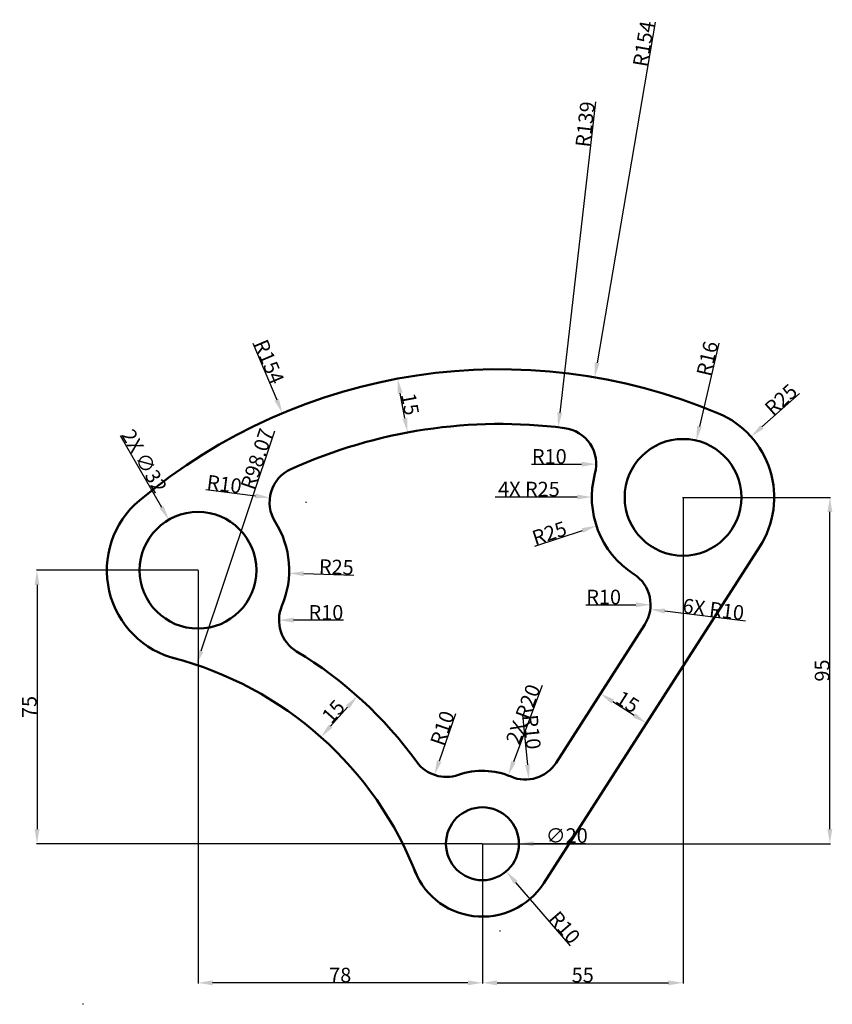
# Model space of a CAD drawing. Units: millimetres. Extents: x 51 to 274, y 49 to 320.
import ezdxf

# ---------------------------------------------------------------- set-up
doc = ezdxf.new("R2010")
doc.units = ezdxf.units.MM
doc.header["$MEASUREMENT"] = 0
doc.layers.add('M-DIMS', color=2, linetype='Continuous', lineweight=25)
doc.layers.add('M-OUTL', color=7, linetype='Continuous', lineweight=50)
doc.styles.get("Standard").update_dxf_attribs({"font": 'arial.ttf'})
doc.dimstyles.get("Standard").update_dxf_attribs({"dimtxt": 4, "dimasz": 4, "dimexe": 0.18, "dimexo": 0.0625, "dimgap": 0.09, "dimtad": 1, "dimdec": 0, "dimzin": 0, "dimdsep": 46, "dimtxsty": 'Standard', "dimcen": 0.09, "dimclre": 251, "dimadec": 0, "dimazin": 0, "dimtfac": 1, "dimtdec": 0, "dimtofl": 0, "dimtmove": 0, "dimatfit": 3, "dimfxl": 1, "dimtolj": 1, "dimtzin": 0, "dimarcsym": 0})

# ---------------------------------------------------------------- blocks, each defined once
blk = doc.blocks.new('*D1')
at = {"layer": 'Defpoints', "color": 0, "transparency": 16777216}
for p in [(233.24, 188.51), (178.24, 93.51), (233.24, 55.36)]:
    blk.add_point(p, dxfattribs=at)
at = {"layer": 'M-DIMS', "color": 0, "lineweight": -2, "transparency": 16777216}
for p, q in [((233.24, 188.45), (233.24, 55.18)), ((178.24, 93.45), (178.24, 55.18)), ((182.24, 55.36), (229.24, 55.36))]:
    blk.add_line(p, q, dxfattribs=at)
at = {"layer": 'M-DIMS', "color": 0, "transparency": 16777216}
for points in [[(182.24, 56.02), (182.24, 54.69), (178.24, 55.36)], [(229.24, 56.02), (229.24, 54.69), (233.24, 55.36)]]:
    blk.add_solid(points, dxfattribs=at)
at = {"layer": 'M-DIMS', "color": 0, "transparency": 16777216, "insert": (205.74, 57.48), "char_height": 4, "attachment_point": 5}
blk.add_mtext('\\A1;55', dxfattribs=at)
blk = doc.blocks.new('*D2')
at = {"layer": 'Defpoints', "color": 0, "transparency": 16777216}
for p in [(100.24, 168.51), (178.24, 93.51), (100.24, 55.36)]:
    blk.add_point(p, dxfattribs=at)
at = {"layer": 'M-DIMS', "color": 0, "lineweight": -2, "transparency": 16777216}
for p, q in [((100.24, 168.45), (100.24, 55.18)), ((178.24, 93.45), (178.24, 55.18)), ((174.24, 55.36), (104.24, 55.36))]:
    blk.add_line(p, q, dxfattribs=at)
at = {"layer": 'M-DIMS', "color": 0, "transparency": 16777216}
for points in [[(104.24, 56.02), (104.24, 54.69), (100.24, 55.36)], [(174.24, 56.02), (174.24, 54.69), (178.24, 55.36)]]:
    blk.add_solid(points, dxfattribs=at)
at = {"layer": 'M-DIMS', "color": 0, "transparency": 16777216, "insert": (139.24, 57.49), "char_height": 4, "attachment_point": 5}
blk.add_mtext('\\A1;78', dxfattribs=at)
blk = doc.blocks.new('*D3')
at = {"layer": 'Defpoints', "color": 0, "transparency": 16777216}
for p in [(233.24, 188.51), (273.51, 188.51), (178.24, 93.51)]:
    blk.add_point(p, dxfattribs=at)
at = {"layer": 'M-DIMS', "color": 0, "lineweight": -2, "transparency": 16777216}
for p, q in [((233.3, 188.51), (273.69, 188.51)), ((273.51, 97.51), (273.51, 184.51)), ((178.3, 93.51), (273.69, 93.51))]:
    blk.add_line(p, q, dxfattribs=at)
at = {"layer": 'M-DIMS', "color": 0, "transparency": 16777216}
for points in [[(272.84, 184.51), (274.18, 184.51), (273.51, 188.51)], [(272.84, 97.51), (274.18, 97.51), (273.51, 93.51)]]:
    blk.add_solid(points, dxfattribs=at)
at = {"layer": 'M-DIMS', "color": 0, "transparency": 16777216, "insert": (271.38, 141.01), "char_height": 4, "attachment_point": 5, "rotation": 90}
blk.add_mtext('\\A1;95', dxfattribs=at)
blk = doc.blocks.new('*D4')
at = {"layer": 'Defpoints', "color": 0, "transparency": 16777216}
for p in [(100.24, 168.51), (56.09, 93.51), (178.24, 93.51)]:
    blk.add_point(p, dxfattribs=at)
at = {"layer": 'M-DIMS', "color": 0, "lineweight": -2, "transparency": 16777216}
for p, q in [((100.18, 168.51), (55.91, 168.51)), ((56.09, 164.51), (56.09, 97.51)), ((178.18, 93.51), (55.91, 93.51))]:
    blk.add_line(p, q, dxfattribs=at)
at = {"layer": 'M-DIMS', "color": 0, "transparency": 16777216}
for points in [[(55.43, 164.51), (56.76, 164.51), (56.09, 168.51)], [(55.43, 97.51), (56.76, 97.51), (56.09, 93.51)]]:
    blk.add_solid(points, dxfattribs=at)
at = {"layer": 'M-DIMS', "color": 0, "transparency": 16777216, "insert": (53.97, 131.01), "char_height": 4, "attachment_point": 5, "rotation": 90}
blk.add_mtext('\\A1;75', dxfattribs=at)
blk = doc.blocks.new('*D5')
at = {"layer": 'Defpoints', "color": 0, "transparency": 16777216}
for p in [(143.92, 133.98), (143.92, 133.98), (133.95, 122.78)]:
    blk.add_point(p, dxfattribs=at)
at = {"layer": 'M-DIMS', "color": 0, "lineweight": -2, "transparency": 16777216}
for p, q in [((143.97, 133.94), (144.06, 133.86)), ((136.61, 125.77), (141.26, 130.99)), ((133.99, 122.74), (134.08, 122.66))]:
    blk.add_line(p, q, dxfattribs=at)
at = {"layer": 'M-DIMS', "color": 0, "transparency": 16777216}
for points in [[(140.77, 131.44), (141.76, 130.55), (143.92, 133.98)], [(136.11, 126.21), (137.11, 125.32), (133.95, 122.78)]]:
    blk.add_solid(points, dxfattribs=at)
at = {"layer": 'M-DIMS', "color": 0, "transparency": 16777216, "insert": (137.34, 129.8), "char_height": 4, "attachment_point": 5, "rotation": 48.3021}
blk.add_mtext('\\A1;15', dxfattribs=at)
blk = doc.blocks.new('*D6')
at = {"layer": 'Defpoints', "color": 0, "transparency": 16777216}
for p in [(154.95, 221.05), (154.95, 221.05), (157.7, 206.31)]:
    blk.add_point(p, dxfattribs=at)
at = {"layer": 'M-DIMS', "color": 0, "lineweight": -2, "transparency": 16777216}
for p, q in [((154.89, 221.04), (154.78, 221.02)), ((156.97, 210.24), (155.69, 217.12)), ((157.64, 206.29), (157.52, 206.27))]:
    blk.add_line(p, q, dxfattribs=at)
at = {"layer": 'M-DIMS', "color": 0, "transparency": 16777216}
for points in [[(156.34, 217.24), (155.03, 217), (154.95, 221.05)], [(157.62, 210.36), (156.31, 210.12), (157.7, 206.31)]]:
    blk.add_solid(points, dxfattribs=at)
at = {"layer": 'M-DIMS', "color": 0, "transparency": 16777216, "insert": (158.42, 214.07), "char_height": 4, "attachment_point": 5, "rotation": 280.5338}
blk.add_mtext('\\A1;15', dxfattribs=at)
blk = doc.blocks.new('*D7')
at = {"layer": 'Defpoints', "color": 0, "transparency": 16777216}
for p in [(210.59, 134.68), (223.21, 126.58), (223.21, 126.58)]:
    blk.add_point(p, dxfattribs=at)
at = {"layer": 'M-DIMS', "color": 0, "lineweight": -2, "transparency": 16777216}
for p, q in [((210.62, 134.73), (210.68, 134.83)), ((213.95, 132.52), (219.85, 128.74)), ((223.25, 126.63), (223.31, 126.73))]:
    blk.add_line(p, q, dxfattribs=at)
at = {"layer": 'M-DIMS', "color": 0, "transparency": 16777216}
for points in [[(214.31, 133.08), (213.59, 131.96), (210.59, 134.68)], [(220.21, 129.3), (219.49, 128.18), (223.21, 126.58)]]:
    blk.add_solid(points, dxfattribs=at)
at = {"layer": 'M-DIMS', "color": 0, "transparency": 16777216, "insert": (218.05, 132.42), "char_height": 4, "attachment_point": 5, "rotation": 327.3208}
blk.add_mtext('\\A1;15', dxfattribs=at)
blk = doc.blocks.new('*D8')
at = {"layer": 'Defpoints', "color": 0, "transparency": 16777216}
for p in [(251.89, 205.15), (233.24, 188.51)]:
    blk.add_point(p, dxfattribs=at)
at = {"layer": 'M-DIMS', "color": 0, "lineweight": -2, "transparency": 16777216}
for p, q in [((265.15, 216.98), (254.88, 207.82)), ((233.15, 188.51), (233.33, 188.51)), ((233.24, 188.42), (233.24, 188.6))]:
    blk.add_line(p, q, dxfattribs=at)
at = {"layer": 'M-DIMS', "color": 0, "transparency": 16777216}
blk.add_solid([(254.43, 208.31), (255.32, 207.32), (251.89, 205.15)], dxfattribs=at)
at = {"layer": 'M-DIMS', "color": 0, "transparency": 16777216, "insert": (260.09, 215.32), "char_height": 4, "attachment_point": 5, "rotation": 41.7376}
blk.add_mtext('\\A1;R25', dxfattribs=at)
blk = doc.blocks.new('*D9')
at = {"layer": 'Defpoints', "color": 0, "transparency": 16777216}
for p in [(236.86, 204.09), (233.24, 188.51)]:
    blk.add_point(p, dxfattribs=at)
at = {"layer": 'M-DIMS', "color": 0, "lineweight": -2, "transparency": 16777216}
for p, q in [((243.07, 230.83), (237.76, 207.99)), ((233.15, 188.51), (233.33, 188.51)), ((233.24, 188.42), (233.24, 188.6))]:
    blk.add_line(p, q, dxfattribs=at)
at = {"layer": 'M-DIMS', "color": 0, "transparency": 16777216}
blk.add_solid([(237.11, 208.14), (238.41, 207.84), (236.86, 204.09)], dxfattribs=at)
at = {"layer": 'M-DIMS', "color": 0, "transparency": 16777216, "insert": (239.89, 226.57), "char_height": 4, "attachment_point": 5, "rotation": 76.92}
blk.add_mtext('\\A1;R16', dxfattribs=at)
blk = doc.blocks.new('*D10')
at = {"layer": 'Defpoints', "color": 0, "transparency": 16777216}
for p in [(233.24, 188.51), (209.49, 180.71)]:
    blk.add_point(p, dxfattribs=at)
at = {"layer": 'M-DIMS', "color": 0, "lineweight": -2, "transparency": 16777216}
for p, q in [((233.15, 188.51), (233.33, 188.51)), ((233.24, 188.42), (233.24, 188.6)), ((192.61, 175.16), (205.69, 179.46))]:
    blk.add_line(p, q, dxfattribs=at)
at = {"layer": 'M-DIMS', "color": 0, "transparency": 16777216}
blk.add_solid([(205.48, 180.09), (205.89, 178.82), (209.49, 180.71)], dxfattribs=at)
at = {"layer": 'M-DIMS', "color": 0, "transparency": 16777216, "insert": (196.58, 178.71), "char_height": 4, "attachment_point": 5, "rotation": 18.1877}
blk.add_mtext('\\A1;R25', dxfattribs=at)
blk = doc.blocks.new('*D11')
at = {"layer": 'Defpoints', "color": 0, "transparency": 16777216}
for p in [(100.24, 168.51), (125.22, 167.7)]:
    blk.add_point(p, dxfattribs=at)
at = {"layer": 'M-DIMS', "color": 0, "lineweight": -2, "transparency": 16777216}
for p, q in [((100.15, 168.51), (100.33, 168.51)), ((100.24, 168.42), (100.24, 168.6)), ((142.98, 167.12), (129.22, 167.57))]:
    blk.add_line(p, q, dxfattribs=at)
at = {"layer": 'M-DIMS', "color": 0, "transparency": 16777216}
blk.add_solid([(129.24, 168.23), (129.2, 166.9), (125.22, 167.7)], dxfattribs=at)
at = {"layer": 'M-DIMS', "color": 0, "transparency": 16777216, "insert": (138.17, 169.41), "char_height": 4, "attachment_point": 5, "rotation": 358.1393}
blk.add_mtext('\\A1;R25', dxfattribs=at)
blk = doc.blocks.new('*D12')
at = {"layer": 'Defpoints', "color": 0, "transparency": 16777216}
for p in [(119.94, 188.41), (129.86, 187.15)]:
    blk.add_point(p, dxfattribs=at)
at = {"layer": 'M-DIMS', "color": 0, "lineweight": -2, "transparency": 16777216}
for p, q in [((102.36, 190.64), (115.97, 188.91)), ((129.77, 187.15), (129.95, 187.15)), ((129.86, 187.06), (129.86, 187.24))]:
    blk.add_line(p, q, dxfattribs=at)
at = {"layer": 'M-DIMS', "color": 0, "transparency": 16777216}
blk.add_solid([(116.06, 189.57), (115.89, 188.25), (119.94, 188.41)], dxfattribs=at)
at = {"layer": 'M-DIMS', "color": 0, "transparency": 16777216, "insert": (107.45, 192.14), "char_height": 4, "attachment_point": 5, "rotation": 352.7636}
blk.add_mtext('\\A1;R10', dxfattribs=at)
blk = doc.blocks.new('*D13')
at = {"layer": 'Defpoints', "color": 0, "transparency": 16777216}
for p in [(199.44, 197.61), (209.44, 197.61)]:
    blk.add_point(p, dxfattribs=at)
at = {"layer": 'M-DIMS', "color": 0, "lineweight": -2, "transparency": 16777216}
blk.add_line((191.72, 197.61), (205.44, 197.61), dxfattribs=at)
at = {"layer": 'M-DIMS', "color": 0, "transparency": 16777216}
blk.add_solid([(205.44, 198.28), (205.44, 196.94), (209.44, 197.61)], dxfattribs=at)
at = {"layer": 'M-DIMS', "color": 0, "transparency": 16777216, "insert": (196.58, 199.74), "char_height": 4, "attachment_point": 5}
blk.add_mtext('\\A1;R10', dxfattribs=at)
blk = doc.blocks.new('*D14')
at = {"layer": 'Defpoints', "color": 0, "transparency": 16777216}
for p in [(214.34, 159.05), (224.34, 159.05)]:
    blk.add_point(p, dxfattribs=at)
at = {"layer": 'M-DIMS', "color": 0, "lineweight": -2, "transparency": 16777216}
blk.add_line((206.62, 159.05), (220.34, 159.05), dxfattribs=at)
at = {"layer": 'M-DIMS', "color": 0, "transparency": 16777216}
blk.add_solid([(220.34, 159.72), (220.34, 158.38), (224.34, 159.05)], dxfattribs=at)
at = {"layer": 'M-DIMS', "color": 0, "transparency": 16777216, "insert": (211.48, 161.18), "char_height": 4, "attachment_point": 5}
blk.add_mtext('\\A1;R10', dxfattribs=at)
blk = doc.blocks.new('*D15')
at = {"layer": 'Defpoints', "color": 0, "transparency": 16777216}
for p in [(190, 121.11), (190.97, 111.15)]:
    blk.add_point(p, dxfattribs=at)
at = {"layer": 'M-DIMS', "color": 0, "lineweight": -2, "transparency": 16777216}
blk.add_line((189.25, 128.8), (190.58, 115.14), dxfattribs=at)
at = {"layer": 'M-DIMS', "color": 0, "transparency": 16777216}
blk.add_solid([(191.24, 115.2), (189.92, 115.07), (190.97, 111.15)], dxfattribs=at)
at = {"layer": 'M-DIMS', "color": 0, "transparency": 16777216, "insert": (191.85, 124.16), "char_height": 4, "attachment_point": 5, "rotation": 275.5492}
blk.add_mtext('\\A1;R10', dxfattribs=at)
blk = doc.blocks.new('*D16')
at = {"layer": 'Defpoints', "color": 0, "transparency": 16777216}
for p in [(168.33, 121.82), (165.08, 112.37)]:
    blk.add_point(p, dxfattribs=at)
at = {"layer": 'M-DIMS', "color": 0, "lineweight": -2, "transparency": 16777216}
blk.add_line((170.84, 129.13), (166.38, 116.15), dxfattribs=at)
at = {"layer": 'M-DIMS', "color": 0, "transparency": 16777216}
blk.add_solid([(165.75, 116.37), (167.01, 115.93), (165.08, 112.37)], dxfattribs=at)
at = {"layer": 'M-DIMS', "color": 0, "transparency": 16777216, "insert": (167.24, 125.22), "char_height": 4, "attachment_point": 5, "rotation": 71.0428}
blk.add_mtext('\\A1;R10', dxfattribs=at)
blk = doc.blocks.new('*D17')
at = {"layer": 'Defpoints', "color": 0, "transparency": 16777216}
for p in [(122.45, 154.83), (132.45, 154.83)]:
    blk.add_point(p, dxfattribs=at)
at = {"layer": 'M-DIMS', "color": 0, "lineweight": -2, "transparency": 16777216}
blk.add_line((140.18, 154.83), (126.45, 154.83), dxfattribs=at)
at = {"layer": 'M-DIMS', "color": 0, "transparency": 16777216}
blk.add_solid([(126.45, 155.5), (126.45, 154.16), (122.45, 154.83)], dxfattribs=at)
at = {"layer": 'M-DIMS', "color": 0, "transparency": 16777216, "insert": (135.32, 156.96), "char_height": 4, "attachment_point": 5}
blk.add_mtext('\\A1;R10', dxfattribs=at)
blk = doc.blocks.new('*D18')
at = {"layer": 'Defpoints', "color": 0, "transparency": 16777216}
for p in [(123.37, 211.59), (183.11, 69.65)]:
    blk.add_point(p, dxfattribs=at)
at = {"layer": 'M-DIMS', "color": 0, "lineweight": -2, "transparency": 16777216}
for p, q in [((115.29, 230.79), (121.82, 215.27)), ((183.02, 69.65), (183.2, 69.65)), ((183.11, 69.56), (183.11, 69.74))]:
    blk.add_line(p, q, dxfattribs=at)
at = {"layer": 'M-DIMS', "color": 0, "transparency": 16777216}
blk.add_solid([(122.43, 215.53), (121.2, 215.02), (123.37, 211.59)], dxfattribs=at)
at = {"layer": 'M-DIMS', "color": 0, "transparency": 16777216, "insert": (119.74, 225.7), "char_height": 4, "attachment_point": 5, "rotation": 292.8258}
blk.add_mtext('\\A1;R154', dxfattribs=at)
blk = doc.blocks.new('*D19')
at = {"layer": 'Defpoints', "color": 0, "transparency": 16777216}
for p in [(178.24, 93.51), (184.75, 85.92)]:
    blk.add_point(p, dxfattribs=at)
at = {"layer": 'M-DIMS', "color": 0, "lineweight": -2, "transparency": 16777216}
for p, q in [((178.15, 93.51), (178.33, 93.51)), ((178.24, 93.42), (178.24, 93.6)), ((202.34, 65.46), (187.36, 82.89))]:
    blk.add_line(p, q, dxfattribs=at)
at = {"layer": 'M-DIMS', "color": 0, "transparency": 16777216}
blk.add_solid([(187.87, 83.32), (186.86, 82.46), (184.75, 85.92)], dxfattribs=at)
at = {"layer": 'M-DIMS', "color": 0, "transparency": 16777216, "insert": (200.79, 70.54), "char_height": 4, "attachment_point": 5, "rotation": 310.6665}
blk.add_mtext('\\A1;R10', dxfattribs=at)
blk = doc.blocks.new('*D20')
at = {"layer": 'Defpoints', "color": 0, "transparency": 16777216}
for p in [(209.01, 221.45), (183.11, 69.65)]:
    blk.add_point(p, dxfattribs=at)
at = {"layer": 'M-DIMS', "color": 0, "lineweight": -2, "transparency": 16777216}
blk.add_line((225.63, 318.86), (209.68, 225.4), dxfattribs=at)
at = {"layer": 'M-DIMS', "color": 251, "lineweight": -2, "transparency": 16777216}
for p, q in [((183.02, 69.65), (183.2, 69.65)), ((183.11, 69.56), (183.11, 69.74))]:
    blk.add_line(p, q, dxfattribs=at)
at = {"layer": 'M-DIMS', "color": 0, "transparency": 16777216}
blk.add_solid([(209.02, 225.51), (210.34, 225.29), (209.01, 221.45)], dxfattribs=at)
at = {"layer": 'M-DIMS', "color": 0, "transparency": 16777216, "insert": (222.45, 312.9), "char_height": 4, "attachment_point": 5, "rotation": 80.3174}
blk.add_mtext('\\A1;R154', dxfattribs=at)
blk = doc.blocks.new('*D21')
at = {"layer": 'Defpoints', "color": 0, "transparency": 16777216}
for p in [(198.99, 207.74), (183.11, 69.65)]:
    blk.add_point(p, dxfattribs=at)
at = {"layer": 'M-DIMS', "color": 0, "lineweight": -2, "transparency": 16777216}
blk.add_line((209.26, 296.98), (199.45, 211.71), dxfattribs=at)
at = {"layer": 'M-DIMS', "color": 251, "lineweight": -2, "transparency": 16777216}
for p, q in [((183.02, 69.65), (183.2, 69.65)), ((183.11, 69.56), (183.11, 69.74))]:
    blk.add_line(p, q, dxfattribs=at)
at = {"layer": 'M-DIMS', "color": 0, "transparency": 16777216}
blk.add_solid([(198.79, 211.79), (200.11, 211.64), (198.99, 207.74)], dxfattribs=at)
at = {"layer": 'M-DIMS', "color": 0, "transparency": 16777216, "insert": (206.4, 290.84), "char_height": 4, "attachment_point": 5, "rotation": 83.438}
blk.add_mtext('\\A1;R139', dxfattribs=at)
blk = doc.blocks.new('*D22')
at = {"layer": 'Defpoints', "color": 0, "transparency": 16777216}
for p in [(99.79, 142.57), (68.71, 49.56)]:
    blk.add_point(p, dxfattribs=at)
at = {"layer": 'M-DIMS', "color": 0, "lineweight": -2, "transparency": 16777216}
blk.add_line((121.21, 206.68), (101.06, 146.36), dxfattribs=at)
at = {"layer": 'M-DIMS', "color": 251, "lineweight": -2, "transparency": 16777216}
for p, q in [((68.62, 49.56), (68.8, 49.56)), ((68.71, 49.47), (68.71, 49.65))]:
    blk.add_line(p, q, dxfattribs=at)
at = {"layer": 'M-DIMS', "color": 0, "transparency": 16777216}
blk.add_solid([(100.43, 146.58), (101.69, 146.15), (99.79, 142.57)], dxfattribs=at)
at = {"layer": 'M-DIMS', "color": 0, "transparency": 16777216, "insert": (116.42, 199.05), "char_height": 4, "attachment_point": 5, "rotation": 71.5237}
blk.add_mtext('\\A1;R98.07', dxfattribs=at)
blk = doc.blocks.new('*D23')
at = {"layer": 'Defpoints', "color": 0, "transparency": 16777216}
for p in [(208.24, 188.6), (233.24, 188.51)]:
    blk.add_point(p, dxfattribs=at)
at = {"layer": 'M-DIMS', "color": 0, "lineweight": -2, "transparency": 16777216}
blk.add_line((181.71, 188.7), (204.24, 188.61), dxfattribs=at)
at = {"layer": 'M-DIMS', "color": 251, "lineweight": -2, "transparency": 16777216}
for p, q in [((233.15, 188.51), (233.33, 188.51)), ((233.24, 188.42), (233.24, 188.6))]:
    blk.add_line(p, q, dxfattribs=at)
at = {"layer": 'M-DIMS', "color": 0, "transparency": 16777216}
blk.add_solid([(204.24, 189.28), (204.24, 187.95), (208.24, 188.6)], dxfattribs=at)
at = {"layer": 'M-DIMS', "color": 0, "transparency": 16777216, "insert": (190.98, 190.79), "char_height": 4, "attachment_point": 5, "rotation": 359.7923}
blk.add_mtext('\\A1;4X R25', dxfattribs=at)
blk = doc.blocks.new('*D24')
at = {"layer": 'Defpoints', "color": 0, "transparency": 16777216}
for p in [(185.31, 112.22), (178.24, 93.51)]:
    blk.add_point(p, dxfattribs=at)
at = {"layer": 'M-DIMS', "color": 0, "lineweight": -2, "transparency": 16777216}
blk.add_line((194.65, 136.9), (186.73, 115.96), dxfattribs=at)
at = {"layer": 'M-DIMS', "color": 251, "lineweight": -2, "transparency": 16777216}
for p, q in [((178.15, 93.51), (178.33, 93.51)), ((178.24, 93.42), (178.24, 93.6))]:
    blk.add_line(p, q, dxfattribs=at)
at = {"layer": 'M-DIMS', "color": 0, "transparency": 16777216}
blk.add_solid([(186.11, 116.19), (187.35, 115.72), (185.31, 112.22)], dxfattribs=at)
at = {"layer": 'M-DIMS', "color": 0, "transparency": 16777216, "insert": (189.4, 129.05), "char_height": 4, "attachment_point": 5, "rotation": 69.2811}
blk.add_mtext('\\A1;2X R20', dxfattribs=at)
blk = doc.blocks.new('*D25')
at = {"layer": 'Defpoints', "color": 0, "transparency": 16777216}
for p in [(214.34, 159.05), (224.26, 157.81)]:
    blk.add_point(p, dxfattribs=at)
at = {"layer": 'M-DIMS', "color": 251, "lineweight": -2, "transparency": 16777216}
for p, q in [((214.25, 159.05), (214.43, 159.05)), ((214.34, 158.96), (214.34, 159.14))]:
    blk.add_line(p, q, dxfattribs=at)
at = {"layer": 'M-DIMS', "color": 0, "lineweight": -2, "transparency": 16777216}
blk.add_line((250.4, 154.56), (228.23, 157.32), dxfattribs=at)
at = {"layer": 'M-DIMS', "color": 0, "transparency": 16777216}
blk.add_solid([(228.32, 157.98), (228.15, 156.66), (224.26, 157.81)], dxfattribs=at)
at = {"layer": 'M-DIMS', "color": 0, "transparency": 16777216, "insert": (241.57, 157.81), "char_height": 4, "attachment_point": 5, "rotation": 352.8996}
blk.add_mtext('\\A1;6X R10', dxfattribs=at)
blk = doc.blocks.new('*D26')
at = {"layer": 'Defpoints', "color": 0, "transparency": 16777216}
for p in [(92.24, 182.37), (108.24, 154.65)]:
    blk.add_point(p, dxfattribs=at)
at = {"layer": 'M-DIMS', "color": 0, "lineweight": -2, "transparency": 16777216}
blk.add_line((78.9, 205.46), (90.24, 185.83), dxfattribs=at)
at = {"layer": 'M-DIMS', "color": 251, "lineweight": -2, "transparency": 16777216}
for p, q in [((100.15, 168.51), (100.33, 168.51)), ((100.24, 168.42), (100.24, 168.6))]:
    blk.add_line(p, q, dxfattribs=at)
at = {"layer": 'M-DIMS', "color": 0, "transparency": 16777216}
blk.add_solid([(90.81, 186.16), (89.66, 185.5), (92.24, 182.37)], dxfattribs=at)
at = {"layer": 'M-DIMS', "color": 0, "transparency": 16777216, "insert": (85.51, 198.5), "char_height": 4, "attachment_point": 5, "rotation": 300.0041}
blk.add_mtext('\\A1;2X ∅32', dxfattribs=at)
blk = doc.blocks.new('*D27')
at = {"layer": 'Defpoints', "color": 0, "transparency": 16777216}
for p in [(168.24, 93.51), (188.24, 93.51)]:
    blk.add_point(p, dxfattribs=at)
at = {"layer": 'M-DIMS', "color": 251, "lineweight": -2, "transparency": 16777216}
for p, q in [((178.15, 93.51), (178.33, 93.51)), ((178.24, 93.42), (178.24, 93.6))]:
    blk.add_line(p, q, dxfattribs=at)
at = {"layer": 'M-DIMS', "color": 0, "lineweight": -2, "transparency": 16777216}
blk.add_line((206.49, 93.51), (192.24, 93.51), dxfattribs=at)
at = {"layer": 'M-DIMS', "color": 0, "transparency": 16777216}
blk.add_solid([(192.24, 94.18), (192.24, 92.84), (188.24, 93.51)], dxfattribs=at)
at = {"layer": 'M-DIMS', "color": 0, "transparency": 16777216, "insert": (201.36, 95.75), "char_height": 4, "attachment_point": 5, "rotation": 359.9976}
blk.add_mtext('\\A1;∅20', dxfattribs=at)

msp = doc.modelspace()

# ---------------------------------------------------------------- linework, layer by layer
at = {"layer": 'M-OUTL'}
for p, q in [((195.072, 82.711), (254.281, 175.011)), ((198.418, 115.708), (222.757, 153.65))]:
    msp.add_line(p, q, dxfattribs=at)
for centre, radius in [((233.238, 188.509), 16), ((100.238, 168.509), 16), ((178.238, 93.509), 10)]:
    msp.add_circle(centre, radius, dxfattribs=at)
for centre, radius, start, end in [((183.108, 69.648), 154, 67.13235, 129.97131), ((233.238, 188.509), 25, 327.32076, 67.13235), ((183.108, 69.648), 139, 82.7258, 114.37786), ((199.442, 197.61), 10, 344.92907, 82.7258), ((129.863, 187.147), 10, 114.37786, 212.17459), ((233.238, 188.509), 25, 164.92907, 237.32076), ((100.238, 168.509), 25, 129.97131, 256.52719), ((100.238, 168.509), 25, 336.99499, 32.17459), ((214.34, 159.05), 10, 327.32076, 57.32076), ((132.454, 154.831), 10, 156.99499, 238.80515), ((68.711, 49.556), 113.069, 35.95987, 58.80515), ((68.711, 49.556), 98.069, 21.09901, 75.50529), ((168.326, 121.825), 10, 215.95987, 289.29211), ((178.238, 93.509), 20, 66.91483, 109.29211), ((190.001, 121.107), 10, 246.91483, 327.32076), ((178.238, 93.509), 20, 198.10442, 327.32076)]:
    msp.add_arc(centre, radius, start, end, dxfattribs=at)

# ---------------------------------------------------------------- dimensions: what is measured, and where the dimension line sits
at = {"layer": 'M-DIMS'}
for center, mpoint, override, picture, middle in [((183.108, 69.648), (209.009, 221.454), {"dimdec": 0, "dimlfac": 1, "dimrnd": 0, "dimzin": 0, "dimdsep": 46, "dimlunit": 2}, '*D20', (224.55, 312.538)), ((183.108, 69.648), (198.993, 207.738), {"dimdec": 0, "dimlfac": 1, "dimrnd": 0, "dimzin": 0, "dimdsep": 46, "dimlunit": 2}, '*D21', (208.524, 290.591)), ((233.238, 188.509), (236.859, 204.094), {"dimclrd": 0, "dimclre": 0, "dimclrt": 0}, '*D9', (241.968, 226.085)), ((68.711, 49.556), (99.79, 142.57), {"dimdec": 2, "dimlfac": 1, "dimrnd": 0, "dimzin": 0, "dimdsep": 46, "dimlunit": 2}, '*D22', (118.438, 198.379)), ((199.442, 197.61), (209.442, 197.61), {"dimclrd": 0, "dimclre": 0, "dimclrt": 0}, '*D13', (196.58, 197.61)), ((214.34, 159.05), (224.34, 159.05), {"dimclrd": 0, "dimclre": 0, "dimclrt": 0}, '*D14', (211.478, 159.05)), ((132.454, 154.831), (122.454, 154.831), {"dimclrd": 0, "dimclre": 0, "dimclrt": 0}, '*D17', (135.317, 154.831)), ((168.326, 121.825), (165.078, 112.367), {"dimclrd": 0, "dimclre": 0, "dimclrt": 0}, '*D16', (169.256, 124.532)), ((190.001, 121.107), (190.968, 111.154), {"dimclrd": 0, "dimclre": 0, "dimclrt": 0}, '*D15', (189.724, 123.956)), ((178.238, 93.509), (184.754, 85.924), {"dimclrd": 0, "dimclre": 0, "dimclrt": 0}, '*D19', (199.168, 69.147))]:
    dim = msp.add_radius_dim(center=center, mpoint=mpoint, dimstyle='Standard', override=override, dxfattribs=at)
    dim.commit()
    dim.dimension.update_dxf_attribs({"geometry": picture, "text_midpoint": middle, "dimtype": 164})
for center, mpoint, picture, middle in [((183.108, 69.648), (123.367, 211.588), '*D18', (119.74, 225.701)), ((233.238, 188.509), (251.893, 205.152), '*D8', (260.088, 215.321)), ((129.863, 187.147), (119.943, 188.407), '*D12', (107.451, 192.142)), ((233.238, 188.509), (209.487, 180.706), '*D10', (196.581, 178.71)), ((100.238, 168.509), (125.225, 167.698), '*D11', (138.171, 169.411))]:
    dim = msp.add_radius_dim(center=center, mpoint=mpoint, dimstyle='Standard', override={"dimclrd": 0, "dimclre": 0, "dimclrt": 0}, dxfattribs=at)
    dim.commit()
    dim.dimension.update_dxf_attribs({"geometry": picture, "text_midpoint": middle})
for p1, p2, picture, middle in [((157.697, 206.306), (154.955, 221.053), '*D6', (158.422, 214.069)), ((210.588, 134.679), (223.213, 126.58), '*D7', (218.052, 132.424)), ((133.947, 122.781), (143.925, 133.981), '*D5', (137.343, 129.799))]:
    dim = msp.add_aligned_dim(p1=p1, p2=p2, distance=0, dimstyle='Standard', override={"dimclrd": 0, "dimclre": 0, "dimclrt": 0}, dxfattribs=at)
    dim.commit()
    dim.dimension.update_dxf_attribs({"geometry": picture, "text_midpoint": middle})
dim = msp.add_diameter_dim_2p(p1=(108.239, 154.654), p2=(92.237, 182.365), text='2X <>', dimstyle='Standard', override={"dimdec": 0, "dimlfac": 1, "dimrnd": 0, "dimzin": 0, "dimdsep": 46, "dimlunit": 2}, dxfattribs=at)
dim.commit()
dim.dimension.update_dxf_attribs({"geometry": '*D26', "text_midpoint": (83.568, 197.378), "dimtype": 163})
for center, mpoint, text, picture, middle in [((233.238, 188.509), (208.238, 188.6), '4X <>', '*D23', (190.984, 190.795)), ((214.34, 159.05), (224.264, 157.814), '6X <>', '*D25', (241.566, 157.807)), ((178.238, 93.509), (185.314, 112.216), '2X <>', '*D24', (189.402, 129.052))]:
    dim = msp.add_radius_dim(center=center, mpoint=mpoint, text=text, dimstyle='Standard', override={"dimdec": 0, "dimlfac": 1, "dimrnd": 0, "dimzin": 0, "dimdsep": 46, "dimlunit": 2}, dxfattribs=at)
    dim.commit()
    dim.dimension.update_dxf_attribs({"geometry": picture, "text_midpoint": middle})
for base, p2, picture, middle in [((233.238, 55.357), (233.238, 188.509), '*D1', (205.738, 57.482)), ((100.238, 55.357), (100.238, 168.509), '*D2', (139.238, 57.49))]:
    dim = msp.add_linear_dim(base=base, p1=(178.238, 93.509), p2=p2, dimstyle='Standard', override={"dimclrd": 0, "dimclre": 0, "dimclrt": 0}, dxfattribs=at)
    dim.commit()
    dim.dimension.update_dxf_attribs({"geometry": picture, "text_midpoint": middle})
for base, p1, p2, picture, middle in [((273.509, 188.509), (178.238, 93.509), (233.238, 188.509), '*D3', (271.377, 141.009)), ((56.092, 93.509), (100.238, 168.509), (178.238, 93.509), '*D4', (53.968, 131.009))]:
    dim = msp.add_linear_dim(base=base, p1=p1, p2=p2, angle=90, dimstyle='Standard', override={"dimclrd": 0, "dimclre": 0, "dimclrt": 0}, dxfattribs=at)
    dim.commit()
    dim.dimension.update_dxf_attribs({"geometry": picture, "text_midpoint": middle})
dim = msp.add_diameter_dim_2p(p1=(168.238, 93.51), p2=(188.238, 93.509), dimstyle='Standard', override={"dimdec": 0, "dimlfac": 1, "dimrnd": 0, "dimzin": 0, "dimdsep": 46, "dimlunit": 2}, dxfattribs=at)
dim.commit()
dim.dimension.update_dxf_attribs({"geometry": '*D27', "text_midpoint": (201.362, 93.508), "dimtype": 163})

doc.saveas('drawing.dxf')
